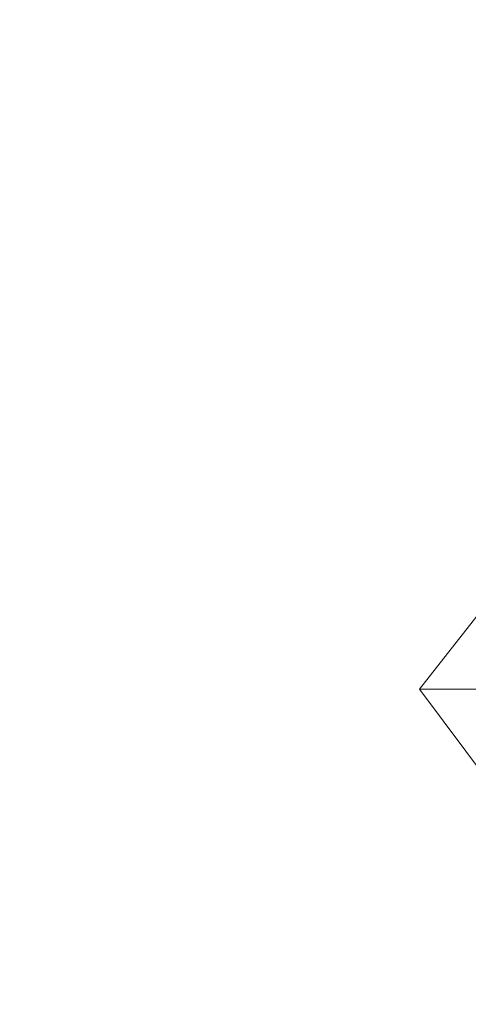
# Model space of a CAD drawing. Units: millimetres. Extents: x 7894 to 8038, y 6851 to 6951.
# Tile 38 of 49: x 7968.188 to 7969.515, y 6925.542 to 6928.457. Entities that reach past the tile are written whole.
import ezdxf

# ---------------------------------------------------------------- set-up
doc = ezdxf.new("R2010")
doc.units = ezdxf.units.MM
doc.layers.add('A-ANNO-DIMS', color=2, linetype='Continuous', lineweight=18)
doc.layers.add('A-FURN-ACCS', color=8, linetype='Continuous', lineweight=13)
doc.styles.get("Standard").update_dxf_attribs({"font": 'arial.ttf'})
doc.dimstyles.new('ISO-25', dxfattribs={"dimtxt": 1, "dimasz": 1, "dimexe": 1.25, "dimexo": 0.625, "dimtad": 1, "dimdec": 0, "dimlunit": 4, "dimtxsty": 'Standard', "dimcen": 2.5, "dimclrt": 1, "dimadec": 0, "dimazin": 0, "dimtfac": 1, "dimtdec": 0, "dimtmove": 0, "dimatfit": 3, "dimfxl": 1, "dimarcsym": 0})

# ---------------------------------------------------------------- blocks, each defined once
blk = doc.blocks.new('DISPLAY-LEAF-FINIAL-Z2_152')
for p, q in [((0, 1.6201, 2.1518), (0.181, 1.8491, 2.1518)), ((0.2072, 1.3429, 2.1518), (0, 1.6201, 2.1518)), ((1.6021, 1.6201, 2.1518), (0, 1.6201, 2.1518))]:
    blk.add_line(p, q)
blk = doc.blocks.new('*D23')
at = {"layer": 'A-ANNO-DIMS', "color": 0, "lineweight": -2, "transparency": 16777216}
for p, q in [((7940.0888, 6907.098), (7940.0888, 6947.7928)), ((7971.9356, 6928.989), (7971.9356, 6947.7928)), ((7941.0888, 6946.5428), (7970.9356, 6946.5428))]:
    blk.add_line(p, q, dxfattribs=at)
at = {"layer": 'A-ANNO-DIMS', "color": 0, "transparency": 16777216}
for points in [[(7941.0888, 6946.7095), (7941.0888, 6946.3762), (7940.0888, 6946.5428)], [(7970.9356, 6946.7095), (7970.9356, 6946.3762), (7971.9356, 6946.5428)]]:
    blk.add_solid(points, dxfattribs=at)
at = {"layer": 'Defpoints', "color": 0, "transparency": 16777216}
for p in [(7971.9356, 6946.5428), (7971.9356, 6928.364), (7940.0888, 6906.473)]:
    blk.add_point(p, dxfattribs=at)
at = {"layer": 'A-ANNO-DIMS', "color": 1, "transparency": 16777216, "insert": (7956.0122, 6947.6784), "char_height": 1, "attachment_point": 5}
blk.add_mtext('2\'-8"', dxfattribs=at)
blk = doc.blocks.new('*D28')
at = {"layer": 'A-ANNO-DIMS', "color": 0, "lineweight": -2, "transparency": 16777216}
for p, q in [((7960.8854, 6936.8804), (7975.2272, 6936.8804)), ((7973.9772, 6935.8804), (7973.9772, 6923.6283)), ((7971.8421, 6922.6283), (7975.2272, 6922.6283))]:
    blk.add_line(p, q, dxfattribs=at)
at = {"layer": 'A-ANNO-DIMS', "color": 0, "transparency": 16777216}
for points in [[(7973.8105, 6935.8804), (7974.1439, 6935.8804), (7973.9772, 6936.8804)], [(7973.8105, 6923.6283), (7974.1439, 6923.6283), (7973.9772, 6922.6283)]]:
    blk.add_solid(points, dxfattribs=at)
at = {"layer": 'Defpoints', "color": 0, "transparency": 16777216}
for p in [(7960.2604, 6936.8804), (7971.2171, 6922.6283), (7973.9772, 6922.6283)]:
    blk.add_point(p, dxfattribs=at)
at = {"layer": 'A-ANNO-DIMS', "color": 1, "transparency": 16777216, "insert": (7972.8351, 6929.7543), "char_height": 1, "attachment_point": 5, "rotation": 90}
blk.add_mtext('1\'-2 1/2"', dxfattribs=at)
blk = doc.blocks.new('*D31')
at = {"layer": 'A-ANNO-DIMS', "color": 0, "lineweight": -2, "transparency": 16777216}
for p, q in [((7973.9772, 6921.7198), (7973.9772, 6926.628)), ((7949.8107, 6920.7198), (7975.2272, 6920.7198)), ((7973.9772, 6918.7198), (7973.9772, 6920.7198)), ((7950.9654, 6918.7198), (7975.2272, 6918.7198)), ((7973.9772, 6917.7198), (7973.9772, 6916.7198))]:
    blk.add_line(p, q, dxfattribs=at)
at = {"layer": 'A-ANNO-DIMS', "color": 0, "transparency": 16777216}
for points in [[(7973.8105, 6921.7198), (7974.1439, 6921.7198), (7973.9772, 6920.7198)], [(7973.8105, 6917.7198), (7974.1439, 6917.7198), (7973.9772, 6918.7198)]]:
    blk.add_solid(points, dxfattribs=at)
at = {"layer": 'Defpoints', "color": 0, "transparency": 16777216}
for p in [(7949.1857, 6920.7198), (7973.9772, 6920.7198), (7950.3404, 6918.7198)]:
    blk.add_point(p, dxfattribs=at)
at = {"layer": 'A-ANNO-DIMS', "color": 1, "transparency": 16777216, "insert": (7972.8416, 6924.6739), "char_height": 1, "attachment_point": 5, "rotation": 90}
blk.add_mtext('0\'-2"', dxfattribs=at)

msp = doc.modelspace()

# ---------------------------------------------------------------- block references
at = {"layer": 'A-FURN-ACCS'}
msp.add_blockref('DISPLAY-LEAF-FINIAL-Z2_152', (7969.3706, 6924.8555), dxfattribs=at)

# ---------------------------------------------------------------- dimensions: what is measured, and where the dimension line sits
at = {"layer": 'A-ANNO-DIMS'}
dim = msp.add_linear_dim(base=(7971.9356, 6946.5428), p1=(7940.0888, 6906.473), p2=(7971.9356, 6928.364), dimstyle='ISO-25', override={"dimdec": 1, "dimlfac": 1, "dimrnd": 0, "dimzin": 1, "dimdsep": 46, "dimlunit": 4, "dimfrac": 2}, dxfattribs=at)
dim.commit()
dim.dimension.update_dxf_attribs({"geometry": '*D23', "text_midpoint": (7956.0122, 6947.6784)})
for base, p1, p2, picture, middle in [((7973.9772, 6922.6283), (7960.2604, 6936.8804), (7971.2171, 6922.6283), '*D28', (7972.8351, 6929.7543)), ((7973.9772, 6920.7198), (7950.3404, 6918.7198), (7949.1857, 6920.7198), '*D31', (7972.8416, 6924.6739))]:
    dim = msp.add_linear_dim(base=base, p1=p1, p2=p2, angle=90, dimstyle='ISO-25', override={"dimdec": 1, "dimlfac": 1, "dimrnd": 0, "dimzin": 1, "dimdsep": 46, "dimlunit": 4, "dimfrac": 2}, dxfattribs=at)
    dim.commit()
    dim.dimension.update_dxf_attribs({"geometry": picture, "text_midpoint": middle})

doc.saveas('drawing.dxf')
